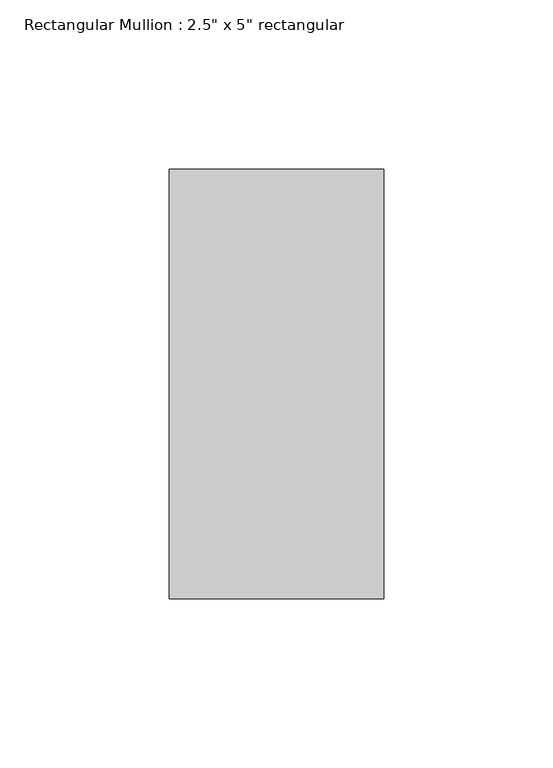
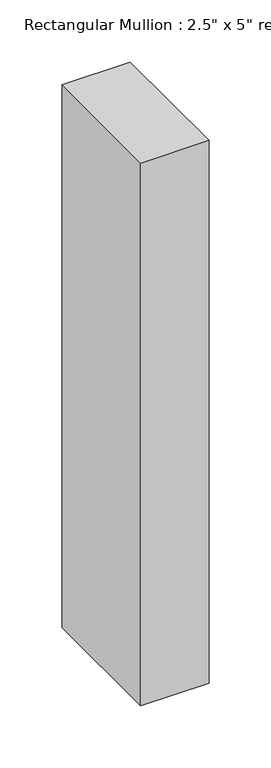
"""IFC4 building model written with IfcOpenShell, lengths in millimetres: member geometry."""

from ifc_helpers import new_model, si_unit, frame, origin, place, context, project, spatial, polyline, outline, extrude, source, transform, mapped, element, save


def member_b281fab0(model_context):
    return source(origin(), model_context, "Body", "SweptSolid", [
        extrude(outline(polyline([(0.0, 63.5), (0.0, -63.5), (-63.5, -63.5), (-63.5, 63.5), (0.0, 63.5)])), frame((0.0, 0.0, -533.4), z_axis=(0.0, 0.0, 1.0), x_axis=(1.0, 0.0, 0.0)), (0.0, 0.0, 1.0), 533.4),
    ])


if __name__ == "__main__":
    model = new_model("IFC4")
    model_context = context("Model", 3, world=origin())
    ifc_project = project(units=[si_unit("LENGTHUNIT", "METRE", prefix="MILLI")], contexts=[model_context])
    site = spatial("IfcSite", under=ifc_project)
    building = spatial("IfcBuilding", under=site)
    placement = place(None, origin())
    member_shape = member_b281fab0(model_context)
    element("IfcMember", 1, ObjectType="Rectangular Mullion : 2.5\" x 5\" rectangular", at=placement, inside=building, context=model_context, shape_type="MappedRepresentation", body=[
        mapped(member_shape, transform((0.0, 0.0, 0.0), x_axis=(1.0, 0.0, 0.0), y_axis=(0.0, 1.0, 0.0), z_axis=(0.0, 0.0, 1.0))),
    ])
    save(model, "model.ifc")

# Revit data of these elements
# Type "Rectangular Mullion : 2.5\" x 5\" rectangular"
#   built-in parameter 1007304 = 0.416667 (stored number, unit not read)
#   built-in parameter 1007301 = 0.104167 (stored number, unit not read)
#   built-in parameter 1007300 = 0.104167 (stored number, unit not read)
# Element 1 (IfcMember, "Rectangular Mullion : 2.5\" x 5\" rectangular")
#   Materials on its faces: "Aluminum"
# Materials
#   "Aluminum": class "Metal", colour RGB 247 247 247, transparency 0, Description = "Aluminum 6061", Cost = 0
